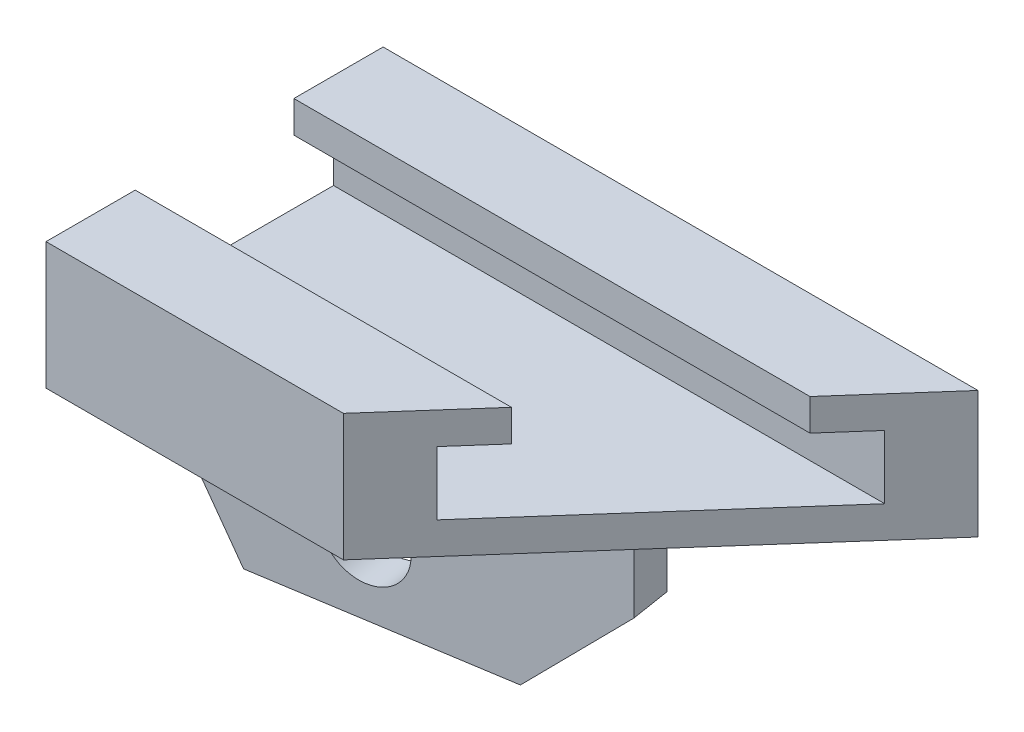
ISO-10303-21;
HEADER;
FILE_DESCRIPTION(('STEP AP214'),'2;1');
FILE_NAME('part.step','',(''),(''),'','','');
FILE_SCHEMA(('AUTOMOTIVE_DESIGN { 1 0 10303 214 1 1 1 1 }'));
ENDSEC;
DATA;
#1=APPLICATION_CONTEXT('core data for automotive mechanical design processes');
#2=APPLICATION_PROTOCOL_DEFINITION('international standard','automotive_design',2000,#1);
#3=PRODUCT_CONTEXT('',#1,'mechanical');
#4=PRODUCT('Part','Part','',(#3));
#5=PRODUCT_RELATED_PRODUCT_CATEGORY('part','',(#4));
#6=PRODUCT_DEFINITION_FORMATION('','',#4);
#7=PRODUCT_DEFINITION_CONTEXT('part definition',#1,'design');
#8=PRODUCT_DEFINITION('design','',#6,#7);
#9=PRODUCT_DEFINITION_SHAPE('','',#8);
#10=(LENGTH_UNIT() NAMED_UNIT(*) SI_UNIT(.MILLI.,.METRE.));
#11=(NAMED_UNIT(*) PLANE_ANGLE_UNIT() SI_UNIT($,.RADIAN.));
#12=(NAMED_UNIT(*) SI_UNIT($,.STERADIAN.) SOLID_ANGLE_UNIT());
#13=UNCERTAINTY_MEASURE_WITH_UNIT(LENGTH_MEASURE(1.E-05),#10,'distance_accuracy_value','');
#14=(GEOMETRIC_REPRESENTATION_CONTEXT(3) GLOBAL_UNCERTAINTY_ASSIGNED_CONTEXT((#13)) GLOBAL_UNIT_ASSIGNED_CONTEXT((#10,
#11,#12)) REPRESENTATION_CONTEXT('',''));
#15=CARTESIAN_POINT('',(0.,0.,0.));
#16=DIRECTION('',(0.,0.,1.));
#17=DIRECTION('',(1.,0.,0.));
#18=AXIS2_PLACEMENT_3D('',#15,#16,#17);
#19=CARTESIAN_POINT('',(32.7590302610631,-40.,-6.27670830561219));
#20=DIRECTION('',(-0.987688340595138,0.,0.156434465040231));
#21=DIRECTION('',(0.156434465040231,0.,0.987688340595138));
#22=AXIS2_PLACEMENT_3D('',#19,#20,#21);
#23=PLANE('',#22);
#24=DIRECTION('',(0.156434465040231,0.,0.987688340595138));
#25=VECTOR('',#24,1.);
#26=CARTESIAN_POINT('',(24.5251727273635,-15.,-58.2632387806263));
#27=LINE('',#26,#25);
#28=CARTESIAN_POINT('',(32.7590302610631,-15.,-6.27670830561219));
#29=VERTEX_POINT('',#28);
#30=CARTESIAN_POINT('',(34.3233749114654,-15.,3.60017510033917));
#31=VERTEX_POINT('',#30);
#32=EDGE_CURVE('E57',#29,#31,#27,.T.);
#33=ORIENTED_EDGE('',*,*,#32,.F.);
#34=DIRECTION('',(0.,1.,0.));
#35=VECTOR('',#34,1.);
#36=CARTESIAN_POINT('',(32.7590302610631,-40.,-6.27670830561219));
#37=LINE('',#36,#35);
#38=CARTESIAN_POINT('',(32.7590302610631,0.,-6.27670830561219));
#39=VERTEX_POINT('',#38);
#40=EDGE_CURVE('E275',#29,#39,#37,.T.);
#41=ORIENTED_EDGE('',*,*,#40,.T.);
#42=DIRECTION('',(0.156434465040231,0.,0.987688340595138));
#43=VECTOR('',#42,1.);
#44=CARTESIAN_POINT('',(32.7590302610631,0.,-6.27670830561219));
#45=LINE('',#44,#43);
#46=CARTESIAN_POINT('',(34.3233749114654,0.,3.60017510033917));
#47=VERTEX_POINT('',#46);
#48=EDGE_CURVE('E188',#39,#47,#45,.T.);
#49=ORIENTED_EDGE('',*,*,#48,.T.);
#50=DIRECTION('',(0.,1.,0.));
#51=VECTOR('',#50,1.);
#52=CARTESIAN_POINT('',(34.3233749114654,-40.,3.60017510033917));
#53=LINE('',#52,#51);
#54=EDGE_CURVE('E400',#31,#47,#53,.T.);
#55=ORIENTED_EDGE('',*,*,#54,.F.);
#56=EDGE_LOOP('',(#33,#41,#49,#55));
#57=FACE_BOUND('',#56,.T.);
#58=ADVANCED_FACE('F39',(#57),#23,.F.);
#59=CARTESIAN_POINT('',(-75.,-40.,10.7906453922011));
#60=DIRECTION('',(0.156434465040231,0.,0.987688340595138));
#61=DIRECTION('',(0.987688340595138,0.,-0.156434465040231));
#62=AXIS2_PLACEMENT_3D('',#59,#60,#61);
#63=PLANE('',#62);
#64=CARTESIAN_POINT('',(-25.6155829702431,-22.,2.96892214018953));
#65=DIRECTION('',(0.156434465040231,0.,0.987688340595138));
#66=DIRECTION('',(0.987688340595138,0.,-0.156434465040231));
#67=AXIS2_PLACEMENT_3D('',#64,#65,#66);
#68=CIRCLE('',#67,10.);
#69=CARTESIAN_POINT('',(-15.7386995642918,-22.,1.40457748978721));
#70=VERTEX_POINT('',#69);
#71=EDGE_CURVE('E190',#70,#70,#68,.T.);
#72=ORIENTED_EDGE('',*,*,#71,.T.);
#73=EDGE_LOOP('',(#72));
#74=FACE_BOUND('',#73,.T.);
#75=ORIENTED_EDGE('',*,*,#40,.F.);
#76=DIRECTION('',(-0.698401123333707,-0.707106781186551,0.110615871041237));
#77=VECTOR('',#76,1.);
#78=CARTESIAN_POINT('',(-33.4665891269071,-82.0511300640304,4.21239935629724));
#79=LINE('',#78,#77);
#80=CARTESIAN_POINT('',(8.06682174618494,-40.,-2.36584667960645));
#81=VERTEX_POINT('',#80);
#82=EDGE_CURVE('E403',#29,#81,#79,.T.);
#83=ORIENTED_EDGE('',*,*,#82,.T.);
#84=DIRECTION('',(0.987688340595138,0.,-0.156434465040231));
#85=VECTOR('',#84,1.);
#86=CARTESIAN_POINT('',(-75.,-40.,10.7906453922011));
#87=LINE('',#86,#85);
#88=CARTESIAN_POINT('',(-52.190314827278,-40.,7.17794617214064));
#89=VERTEX_POINT('',#88);
#90=EDGE_CURVE('E167',#89,#81,#87,.T.);
#91=ORIENTED_EDGE('',*,*,#90,.F.);
#92=DIRECTION('',(0.493844170297564,-0.866025403784441,-0.0782172325201147));
#93=VECTOR('',#92,1.);
#94=CARTESIAN_POINT('',(-57.8927361204584,-30.0000000000002,8.08112097715573));
#95=LINE('',#94,#93);
#96=CARTESIAN_POINT('',(-75.,0.,10.7906453922011));
#97=VERTEX_POINT('',#96);
#98=EDGE_CURVE('E159',#97,#89,#95,.T.);
#99=ORIENTED_EDGE('',*,*,#98,.F.);
#100=DIRECTION('',(0.987688340595138,0.,-0.156434465040231));
#101=VECTOR('',#100,1.);
#102=CARTESIAN_POINT('',(-75.,0.,10.7906453922011));
#103=LINE('',#102,#101);
#104=EDGE_CURVE('E175',#97,#39,#103,.T.);
#105=ORIENTED_EDGE('',*,*,#104,.T.);
#106=EDGE_LOOP('',(#75,#83,#91,#99,#105));
#107=FACE_BOUND('',#106,.T.);
#108=ADVANCED_FACE('F173',(#74,#107),#63,.F.);
#109=CARTESIAN_POINT('',(-73.4356553495977,-40.,20.6675287981525));
#110=DIRECTION('',(-0.156434465040231,0.,-0.987688340595138));
#111=DIRECTION('',(-0.987688340595138,0.,0.156434465040231));
#112=AXIS2_PLACEMENT_3D('',#109,#110,#111);
#113=PLANE('',#112);
#114=CARTESIAN_POINT('',(-24.0512383198408,-22.,12.8458055461409));
#115=DIRECTION('',(-0.156434465040231,0.,-0.987688340595138));
#116=DIRECTION('',(-0.987688340595138,0.,0.156434465040231));
#117=AXIS2_PLACEMENT_3D('',#114,#115,#116);
#118=CIRCLE('',#117,10.);
#119=CARTESIAN_POINT('',(-33.9281217257922,-22.,14.4101501965432));
#120=VERTEX_POINT('',#119);
#121=EDGE_CURVE('E43',#120,#120,#118,.T.);
#122=ORIENTED_EDGE('',*,*,#121,.T.);
#123=EDGE_LOOP('',(#122));
#124=FACE_BOUND('',#123,.T.);
#125=DIRECTION('',(-0.987688340595138,0.,0.156434465040231));
#126=VECTOR('',#125,1.);
#127=CARTESIAN_POINT('',(-73.4356553495977,-40.,20.6675287981525));
#128=LINE('',#127,#126);
#129=CARTESIAN_POINT('',(9.63116639658725,-40.,7.51103672634494));
#130=VERTEX_POINT('',#129);
#131=CARTESIAN_POINT('',(-50.6259701768757,-40.,17.054829578092));
#132=VERTEX_POINT('',#131);
#133=EDGE_CURVE('E395',#130,#132,#128,.T.);
#134=ORIENTED_EDGE('',*,*,#133,.F.);
#135=DIRECTION('',(0.698401123333707,0.707106781186551,-0.110615871041237));
#136=VECTOR('',#135,1.);
#137=CARTESIAN_POINT('',(-31.9022444765048,-82.0511300640304,14.0892827622486));
#138=LINE('',#137,#136);
#139=EDGE_CURVE('E177',#130,#31,#138,.T.);
#140=ORIENTED_EDGE('',*,*,#139,.T.);
#141=ORIENTED_EDGE('',*,*,#54,.T.);
#142=DIRECTION('',(-0.987688340595138,0.,0.156434465040231));
#143=VECTOR('',#142,1.);
#144=CARTESIAN_POINT('',(-73.4356553495977,0.,20.6675287981525));
#145=LINE('',#144,#143);
#146=CARTESIAN_POINT('',(-73.4356553495977,0.,20.6675287981525));
#147=VERTEX_POINT('',#146);
#148=EDGE_CURVE('E170',#47,#147,#145,.T.);
#149=ORIENTED_EDGE('',*,*,#148,.T.);
#150=DIRECTION('',(-0.493844170297564,0.866025403784442,0.0782172325201148));
#151=VECTOR('',#150,1.);
#152=CARTESIAN_POINT('',(-56.3283914700561,-30.0000000000002,17.9580043831071));
#153=LINE('',#152,#151);
#154=EDGE_CURVE('E161',#132,#147,#153,.T.);
#155=ORIENTED_EDGE('',*,*,#154,.F.);
#156=EDGE_LOOP('',(#134,#140,#141,#149,#155));
#157=FACE_BOUND('',#156,.T.);
#158=ADVANCED_FACE('F355',(#124,#157),#113,.F.);
#159=CARTESIAN_POINT('',(0.,-40.,0.));
#160=DIRECTION('',(0.,-1.,0.));
#161=DIRECTION('',(0.,0.,-1.));
#162=AXIS2_PLACEMENT_3D('',#159,#160,#161);
#163=PLANE('',#162);
#164=ORIENTED_EDGE('',*,*,#90,.T.);
#165=DIRECTION('',(0.156434465040231,0.,0.987688340595138));
#166=VECTOR('',#165,1.);
#167=CARTESIAN_POINT('',(-0.167035787514648,-40.,-54.3523771546206));
#168=LINE('',#167,#166);
#169=EDGE_CURVE('E11',#81,#130,#168,.T.);
#170=ORIENTED_EDGE('',*,*,#169,.T.);
#171=ORIENTED_EDGE('',*,*,#133,.T.);
#172=DIRECTION('',(0.156434465040231,0.,0.987688340595138));
#173=VECTOR('',#172,1.);
#174=CARTESIAN_POINT('',(-60.4241723609776,-40.,-44.8085843028735));
#175=LINE('',#174,#173);
#176=EDGE_CURVE('E48',#89,#132,#175,.T.);
#177=ORIENTED_EDGE('',*,*,#176,.F.);
#178=EDGE_LOOP('',(#164,#170,#171,#177));
#179=FACE_BOUND('',#178,.T.);
#180=ADVANCED_FACE('F383',(#179),#163,.T.);
#181=CARTESIAN_POINT('',(0.,0.,0.));
#182=DIRECTION('',(0.,1.,0.));
#183=DIRECTION('',(0.,0.,1.));
#184=AXIS2_PLACEMENT_3D('',#181,#182,#183);
#185=PLANE('',#184);
#186=ORIENTED_EDGE('',*,*,#104,.F.);
#187=DIRECTION('',(0.,0.,1.));
#188=VECTOR('',#187,1.);
#189=CARTESIAN_POINT('',(-75.,0.,-42.5));
#190=LINE('',#189,#188);
#191=CARTESIAN_POINT('',(-75.,0.,-42.5));
#192=VERTEX_POINT('',#191);
#193=EDGE_CURVE('E186',#192,#97,#190,.T.);
#194=ORIENTED_EDGE('',*,*,#193,.F.);
#195=DIRECTION('',(-1.,0.,0.));
#196=VECTOR('',#195,1.);
#197=CARTESIAN_POINT('',(-75.,0.,-42.5));
#198=LINE('',#197,#196);
#199=CARTESIAN_POINT('',(75.,0.,-42.5));
#200=VERTEX_POINT('',#199);
#201=EDGE_CURVE('E216',#200,#192,#198,.T.);
#202=ORIENTED_EDGE('',*,*,#201,.F.);
#203=DIRECTION('',(0.661621637086846,0.,-0.749837855365093));
#204=VECTOR('',#203,1.);
#205=CARTESIAN_POINT('',(0.,0.,42.5));
#206=LINE('',#205,#204);
#207=EDGE_CURVE('E210',#47,#200,#206,.T.);
#208=ORIENTED_EDGE('',*,*,#207,.F.);
#209=ORIENTED_EDGE('',*,*,#48,.F.);
#210=EDGE_LOOP('',(#186,#194,#202,#208,#209));
#211=FACE_BOUND('',#210,.T.);
#212=ADVANCED_FACE('F181',(#211),#185,.F.);
#213=DIRECTION('',(-0.156434465040231,0.,-0.987688340595138));
#214=VECTOR('',#213,1.);
#215=CARTESIAN_POINT('',(-75.,0.,10.7906453922011));
#216=LINE('',#215,#214);
#217=EDGE_CURVE('E160',#147,#97,#216,.T.);
#218=ORIENTED_EDGE('',*,*,#217,.F.);
#219=ORIENTED_EDGE('',*,*,#148,.F.);
#220=CARTESIAN_POINT('',(0.,0.,42.5));
#221=VERTEX_POINT('',#220);
#222=EDGE_CURVE('E213',#221,#47,#206,.T.);
#223=ORIENTED_EDGE('',*,*,#222,.F.);
#224=DIRECTION('',(1.,0.,0.));
#225=VECTOR('',#224,1.);
#226=CARTESIAN_POINT('',(-75.,0.,42.5));
#227=LINE('',#226,#225);
#228=CARTESIAN_POINT('',(-75.,0.,42.5));
#229=VERTEX_POINT('',#228);
#230=EDGE_CURVE('E198',#229,#221,#227,.T.);
#231=ORIENTED_EDGE('',*,*,#230,.F.);
#232=EDGE_CURVE('E192',#97,#229,#190,.T.);
#233=ORIENTED_EDGE('',*,*,#232,.F.);
#234=EDGE_LOOP('',(#218,#219,#223,#231,#233));
#235=FACE_BOUND('',#234,.T.);
#236=ADVANCED_FACE('F193',(#235),#185,.F.);
#237=CARTESIAN_POINT('',(-75.,32.,-42.5));
#238=DIRECTION('',(1.,0.,0.));
#239=DIRECTION('',(0.,0.,-1.));
#240=AXIS2_PLACEMENT_3D('',#237,#238,#239);
#241=PLANE('',#240);
#242=DIRECTION('',(0.,1.,0.));
#243=VECTOR('',#242,1.);
#244=CARTESIAN_POINT('',(-75.,32.,20.));
#245=LINE('',#244,#243);
#246=CARTESIAN_POINT('',(-75.,24.,20.));
#247=VERTEX_POINT('',#246);
#248=CARTESIAN_POINT('',(-75.,32.,20.));
#249=VERTEX_POINT('',#248);
#250=EDGE_CURVE('E270',#247,#249,#245,.T.);
#251=ORIENTED_EDGE('',*,*,#250,.F.);
#252=DIRECTION('',(0.,0.,-1.));
#253=VECTOR('',#252,1.);
#254=CARTESIAN_POINT('',(-75.,24.,20.));
#255=LINE('',#254,#253);
#256=CARTESIAN_POINT('',(-75.,24.,30.));
#257=VERTEX_POINT('',#256);
#258=EDGE_CURVE('E267',#257,#247,#255,.T.);
#259=ORIENTED_EDGE('',*,*,#258,.F.);
#260=DIRECTION('',(0.,1.,0.));
#261=VECTOR('',#260,1.);
#262=CARTESIAN_POINT('',(-75.,8.,30.));
#263=LINE('',#262,#261);
#264=CARTESIAN_POINT('',(-75.,8.,30.));
#265=VERTEX_POINT('',#264);
#266=EDGE_CURVE('E253',#265,#257,#263,.T.);
#267=ORIENTED_EDGE('',*,*,#266,.F.);
#268=DIRECTION('',(0.,0.,1.));
#269=VECTOR('',#268,1.);
#270=CARTESIAN_POINT('',(-75.,8.,-30.));
#271=LINE('',#270,#269);
#272=CARTESIAN_POINT('',(-75.,8.,-30.));
#273=VERTEX_POINT('',#272);
#274=EDGE_CURVE('E254',#273,#265,#271,.T.);
#275=ORIENTED_EDGE('',*,*,#274,.F.);
#276=DIRECTION('',(0.,-1.,0.));
#277=VECTOR('',#276,1.);
#278=CARTESIAN_POINT('',(-75.,8.,-30.));
#279=LINE('',#278,#277);
#280=CARTESIAN_POINT('',(-75.,24.,-30.));
#281=VERTEX_POINT('',#280);
#282=EDGE_CURVE('E256',#281,#273,#279,.T.);
#283=ORIENTED_EDGE('',*,*,#282,.F.);
#284=DIRECTION('',(0.,0.,-1.));
#285=VECTOR('',#284,1.);
#286=CARTESIAN_POINT('',(-75.,24.,-30.));
#287=LINE('',#286,#285);
#288=CARTESIAN_POINT('',(-75.,24.,-20.));
#289=VERTEX_POINT('',#288);
#290=EDGE_CURVE('E261',#289,#281,#287,.T.);
#291=ORIENTED_EDGE('',*,*,#290,.F.);
#292=DIRECTION('',(0.,-1.,0.));
#293=VECTOR('',#292,1.);
#294=CARTESIAN_POINT('',(-75.,32.,-20.));
#295=LINE('',#294,#293);
#296=CARTESIAN_POINT('',(-75.,32.,-20.));
#297=VERTEX_POINT('',#296);
#298=EDGE_CURVE('E262',#297,#289,#295,.T.);
#299=ORIENTED_EDGE('',*,*,#298,.F.);
#300=DIRECTION('',(0.,0.,1.));
#301=VECTOR('',#300,1.);
#302=CARTESIAN_POINT('',(-75.,32.,0.));
#303=LINE('',#302,#301);
#304=CARTESIAN_POINT('',(-75.,32.,-42.5));
#305=VERTEX_POINT('',#304);
#306=EDGE_CURVE('E235',#305,#297,#303,.T.);
#307=ORIENTED_EDGE('',*,*,#306,.F.);
#308=DIRECTION('',(0.,-1.,0.));
#309=VECTOR('',#308,1.);
#310=CARTESIAN_POINT('',(-75.,32.,-42.5));
#311=LINE('',#310,#309);
#312=EDGE_CURVE('E206',#305,#192,#311,.T.);
#313=ORIENTED_EDGE('',*,*,#312,.T.);
#314=ORIENTED_EDGE('',*,*,#193,.T.);
#315=ORIENTED_EDGE('',*,*,#232,.T.);
#316=DIRECTION('',(0.,-1.,0.));
#317=VECTOR('',#316,1.);
#318=CARTESIAN_POINT('',(-75.,32.,42.5));
#319=LINE('',#318,#317);
#320=CARTESIAN_POINT('',(-75.,32.,42.5));
#321=VERTEX_POINT('',#320);
#322=EDGE_CURVE('E223',#321,#229,#319,.T.);
#323=ORIENTED_EDGE('',*,*,#322,.F.);
#324=DIRECTION('',(0.,0.,1.));
#325=VECTOR('',#324,1.);
#326=CARTESIAN_POINT('',(-75.,32.,0.));
#327=LINE('',#326,#325);
#328=EDGE_CURVE('E217',#249,#321,#327,.T.);
#329=ORIENTED_EDGE('',*,*,#328,.F.);
#330=EDGE_LOOP('',(#251,#259,#267,#275,#283,#291,#299,#307,#313,#314,#315,#323,#329));
#331=FACE_BOUND('',#330,.T.);
#332=ADVANCED_FACE('F41',(#331),#241,.F.);
#333=CARTESIAN_POINT('',(0.,32.,0.));
#334=DIRECTION('',(0.,1.,0.));
#335=DIRECTION('',(0.,0.,1.));
#336=AXIS2_PLACEMENT_3D('',#333,#334,#335);
#337=PLANE('',#336);
#338=DIRECTION('',(0.661621637086846,0.,-0.749837855365093));
#339=VECTOR('',#338,1.);
#340=CARTESIAN_POINT('',(0.,32.,42.5));
#341=LINE('',#340,#339);
#342=CARTESIAN_POINT('',(0.,32.,42.5));
#343=VERTEX_POINT('',#342);
#344=CARTESIAN_POINT('',(19.8529411764706,32.,20.));
#345=VERTEX_POINT('',#344);
#346=EDGE_CURVE('E209',#343,#345,#341,.T.);
#347=ORIENTED_EDGE('',*,*,#346,.T.);
#348=DIRECTION('',(-1.,0.,0.));
#349=VECTOR('',#348,1.);
#350=CARTESIAN_POINT('',(75.,32.,20.));
#351=LINE('',#350,#349);
#352=EDGE_CURVE('E233',#345,#249,#351,.T.);
#353=ORIENTED_EDGE('',*,*,#352,.T.);
#354=ORIENTED_EDGE('',*,*,#328,.T.);
#355=DIRECTION('',(1.,0.,0.));
#356=VECTOR('',#355,1.);
#357=CARTESIAN_POINT('',(-75.,32.,42.5));
#358=LINE('',#357,#356);
#359=EDGE_CURVE('E228',#321,#343,#358,.T.);
#360=ORIENTED_EDGE('',*,*,#359,.T.);
#361=EDGE_LOOP('',(#347,#353,#354,#360));
#362=FACE_BOUND('',#361,.T.);
#363=ADVANCED_FACE('F276',(#362),#337,.T.);
#364=CARTESIAN_POINT('',(-75.,32.,42.5));
#365=DIRECTION('',(0.,0.,-1.));
#366=DIRECTION('',(-1.,0.,0.));
#367=AXIS2_PLACEMENT_3D('',#364,#365,#366);
#368=PLANE('',#367);
#369=ORIENTED_EDGE('',*,*,#230,.T.);
#370=DIRECTION('',(0.,-1.,0.));
#371=VECTOR('',#370,1.);
#372=CARTESIAN_POINT('',(0.,32.,42.5));
#373=LINE('',#372,#371);
#374=EDGE_CURVE('E225',#343,#221,#373,.T.);
#375=ORIENTED_EDGE('',*,*,#374,.F.);
#376=ORIENTED_EDGE('',*,*,#359,.F.);
#377=ORIENTED_EDGE('',*,*,#322,.T.);
#378=EDGE_LOOP('',(#369,#375,#376,#377));
#379=FACE_BOUND('',#378,.T.);
#380=ADVANCED_FACE('F282',(#379),#368,.F.);
#381=CARTESIAN_POINT('',(0.,32.,42.5));
#382=DIRECTION('',(-0.749837855365093,0.,-0.661621637086846));
#383=DIRECTION('',(-0.661621637086846,0.,0.749837855365093));
#384=AXIS2_PLACEMENT_3D('',#381,#382,#383);
#385=PLANE('',#384);
#386=CARTESIAN_POINT('',(55.1470588235294,32.,-20.));
#387=VERTEX_POINT('',#386);
#388=CARTESIAN_POINT('',(75.,32.,-42.5));
#389=VERTEX_POINT('',#388);
#390=EDGE_CURVE('E231',#387,#389,#341,.T.);
#391=ORIENTED_EDGE('',*,*,#390,.F.);
#392=DIRECTION('',(0.,-1.,0.));
#393=VECTOR('',#392,1.);
#394=CARTESIAN_POINT('',(55.1470588235294,32.,-20.));
#395=LINE('',#394,#393);
#396=CARTESIAN_POINT('',(55.1470588235294,24.,-20.));
#397=VERTEX_POINT('',#396);
#398=EDGE_CURVE('E199',#387,#397,#395,.T.);
#399=ORIENTED_EDGE('',*,*,#398,.T.);
#400=DIRECTION('',(0.661621637086846,0.,-0.749837855365093));
#401=VECTOR('',#400,1.);
#402=CARTESIAN_POINT('',(0.,24.,42.5));
#403=LINE('',#402,#401);
#404=CARTESIAN_POINT('',(63.9705882352941,24.,-30.));
#405=VERTEX_POINT('',#404);
#406=EDGE_CURVE('E247',#397,#405,#403,.T.);
#407=ORIENTED_EDGE('',*,*,#406,.T.);
#408=DIRECTION('',(0.,-1.,0.));
#409=VECTOR('',#408,1.);
#410=CARTESIAN_POINT('',(63.9705882352941,32.,-30.));
#411=LINE('',#410,#409);
#412=CARTESIAN_POINT('',(63.9705882352941,8.,-30.));
#413=VERTEX_POINT('',#412);
#414=EDGE_CURVE('E245',#405,#413,#411,.T.);
#415=ORIENTED_EDGE('',*,*,#414,.T.);
#416=DIRECTION('',(-0.661621637086846,0.,0.749837855365093));
#417=VECTOR('',#416,1.);
#418=CARTESIAN_POINT('',(0.,8.,42.5));
#419=LINE('',#418,#417);
#420=CARTESIAN_POINT('',(11.0294117647059,8.,30.));
#421=VERTEX_POINT('',#420);
#422=EDGE_CURVE('E242',#413,#421,#419,.T.);
#423=ORIENTED_EDGE('',*,*,#422,.T.);
#424=DIRECTION('',(0.,1.,0.));
#425=VECTOR('',#424,1.);
#426=CARTESIAN_POINT('',(11.0294117647059,32.,30.));
#427=LINE('',#426,#425);
#428=CARTESIAN_POINT('',(11.0294117647059,24.,30.));
#429=VERTEX_POINT('',#428);
#430=EDGE_CURVE('E236',#421,#429,#427,.T.);
#431=ORIENTED_EDGE('',*,*,#430,.T.);
#432=DIRECTION('',(0.661621637086846,0.,-0.749837855365093));
#433=VECTOR('',#432,1.);
#434=CARTESIAN_POINT('',(0.,24.,42.5));
#435=LINE('',#434,#433);
#436=CARTESIAN_POINT('',(19.8529411764706,24.,20.));
#437=VERTEX_POINT('',#436);
#438=EDGE_CURVE('E234',#429,#437,#435,.T.);
#439=ORIENTED_EDGE('',*,*,#438,.T.);
#440=DIRECTION('',(0.,1.,0.));
#441=VECTOR('',#440,1.);
#442=CARTESIAN_POINT('',(19.8529411764706,32.,20.));
#443=LINE('',#442,#441);
#444=EDGE_CURVE('E287',#437,#345,#443,.T.);
#445=ORIENTED_EDGE('',*,*,#444,.T.);
#446=ORIENTED_EDGE('',*,*,#346,.F.);
#447=ORIENTED_EDGE('',*,*,#374,.T.);
#448=ORIENTED_EDGE('',*,*,#222,.T.);
#449=ORIENTED_EDGE('',*,*,#207,.T.);
#450=DIRECTION('',(0.,-1.,0.));
#451=VECTOR('',#450,1.);
#452=CARTESIAN_POINT('',(75.,32.,-42.5));
#453=LINE('',#452,#451);
#454=EDGE_CURVE('E218',#389,#200,#453,.T.);
#455=ORIENTED_EDGE('',*,*,#454,.F.);
#456=EDGE_LOOP('',(#391,#399,#407,#415,#423,#431,#439,#445,#446,#447,#448,#449,#455));
#457=FACE_BOUND('',#456,.T.);
#458=ADVANCED_FACE('F290',(#457),#385,.F.);
#459=CARTESIAN_POINT('',(-75.,32.,-42.5));
#460=DIRECTION('',(0.,0.,1.));
#461=DIRECTION('',(1.,0.,0.));
#462=AXIS2_PLACEMENT_3D('',#459,#460,#461);
#463=PLANE('',#462);
#464=ORIENTED_EDGE('',*,*,#201,.T.);
#465=ORIENTED_EDGE('',*,*,#312,.F.);
#466=DIRECTION('',(-1.,0.,0.));
#467=VECTOR('',#466,1.);
#468=CARTESIAN_POINT('',(-75.,32.,-42.5));
#469=LINE('',#468,#467);
#470=EDGE_CURVE('E226',#389,#305,#469,.T.);
#471=ORIENTED_EDGE('',*,*,#470,.F.);
#472=ORIENTED_EDGE('',*,*,#454,.T.);
#473=EDGE_LOOP('',(#464,#465,#471,#472));
#474=FACE_BOUND('',#473,.T.);
#475=ADVANCED_FACE('F296',(#474),#463,.F.);
#476=DIRECTION('',(-1.,0.,0.));
#477=VECTOR('',#476,1.);
#478=CARTESIAN_POINT('',(75.,32.,-20.));
#479=LINE('',#478,#477);
#480=EDGE_CURVE('E239',#387,#297,#479,.T.);
#481=ORIENTED_EDGE('',*,*,#480,.F.);
#482=ORIENTED_EDGE('',*,*,#390,.T.);
#483=ORIENTED_EDGE('',*,*,#470,.T.);
#484=ORIENTED_EDGE('',*,*,#306,.T.);
#485=EDGE_LOOP('',(#481,#482,#483,#484));
#486=FACE_BOUND('',#485,.T.);
#487=ADVANCED_FACE('F295',(#486),#337,.T.);
#488=CARTESIAN_POINT('',(75.,24.,20.));
#489=DIRECTION('',(0.,1.,0.));
#490=DIRECTION('',(0.,0.,1.));
#491=AXIS2_PLACEMENT_3D('',#488,#489,#490);
#492=PLANE('',#491);
#493=DIRECTION('',(-1.,0.,0.));
#494=VECTOR('',#493,1.);
#495=CARTESIAN_POINT('',(75.,24.,30.));
#496=LINE('',#495,#494);
#497=EDGE_CURVE('E312',#429,#257,#496,.T.);
#498=ORIENTED_EDGE('',*,*,#497,.T.);
#499=ORIENTED_EDGE('',*,*,#258,.T.);
#500=DIRECTION('',(-1.,0.,0.));
#501=VECTOR('',#500,1.);
#502=CARTESIAN_POINT('',(75.,24.,20.));
#503=LINE('',#502,#501);
#504=EDGE_CURVE('E255',#437,#247,#503,.T.);
#505=ORIENTED_EDGE('',*,*,#504,.F.);
#506=ORIENTED_EDGE('',*,*,#438,.F.);
#507=EDGE_LOOP('',(#498,#499,#505,#506));
#508=FACE_BOUND('',#507,.T.);
#509=ADVANCED_FACE('F339',(#508),#492,.F.);
#510=CARTESIAN_POINT('',(75.,8.,30.));
#511=DIRECTION('',(0.,0.,1.));
#512=DIRECTION('',(1.,0.,0.));
#513=AXIS2_PLACEMENT_3D('',#510,#511,#512);
#514=PLANE('',#513);
#515=DIRECTION('',(-1.,0.,0.));
#516=VECTOR('',#515,1.);
#517=CARTESIAN_POINT('',(75.,8.,30.));
#518=LINE('',#517,#516);
#519=EDGE_CURVE('E311',#421,#265,#518,.T.);
#520=ORIENTED_EDGE('',*,*,#519,.T.);
#521=ORIENTED_EDGE('',*,*,#266,.T.);
#522=ORIENTED_EDGE('',*,*,#497,.F.);
#523=ORIENTED_EDGE('',*,*,#430,.F.);
#524=EDGE_LOOP('',(#520,#521,#522,#523));
#525=FACE_BOUND('',#524,.T.);
#526=ADVANCED_FACE('F328',(#525),#514,.F.);
#527=CARTESIAN_POINT('',(75.,8.,-30.));
#528=DIRECTION('',(0.,-1.,0.));
#529=DIRECTION('',(0.,0.,-1.));
#530=AXIS2_PLACEMENT_3D('',#527,#528,#529);
#531=PLANE('',#530);
#532=DIRECTION('',(-1.,0.,0.));
#533=VECTOR('',#532,1.);
#534=CARTESIAN_POINT('',(75.,8.,-30.));
#535=LINE('',#534,#533);
#536=EDGE_CURVE('E313',#413,#273,#535,.T.);
#537=ORIENTED_EDGE('',*,*,#536,.T.);
#538=ORIENTED_EDGE('',*,*,#274,.T.);
#539=ORIENTED_EDGE('',*,*,#519,.F.);
#540=ORIENTED_EDGE('',*,*,#422,.F.);
#541=EDGE_LOOP('',(#537,#538,#539,#540));
#542=FACE_BOUND('',#541,.T.);
#543=ADVANCED_FACE('F322',(#542),#531,.F.);
#544=CARTESIAN_POINT('',(75.,8.,-30.));
#545=DIRECTION('',(0.,0.,-1.));
#546=DIRECTION('',(-1.,0.,0.));
#547=AXIS2_PLACEMENT_3D('',#544,#545,#546);
#548=PLANE('',#547);
#549=DIRECTION('',(-1.,0.,0.));
#550=VECTOR('',#549,1.);
#551=CARTESIAN_POINT('',(75.,24.,-30.));
#552=LINE('',#551,#550);
#553=EDGE_CURVE('E310',#405,#281,#552,.T.);
#554=ORIENTED_EDGE('',*,*,#553,.T.);
#555=ORIENTED_EDGE('',*,*,#282,.T.);
#556=ORIENTED_EDGE('',*,*,#536,.F.);
#557=ORIENTED_EDGE('',*,*,#414,.F.);
#558=EDGE_LOOP('',(#554,#555,#556,#557));
#559=FACE_BOUND('',#558,.T.);
#560=ADVANCED_FACE('F319',(#559),#548,.F.);
#561=CARTESIAN_POINT('',(75.,24.,-30.));
#562=DIRECTION('',(0.,1.,0.));
#563=DIRECTION('',(0.,0.,1.));
#564=AXIS2_PLACEMENT_3D('',#561,#562,#563);
#565=PLANE('',#564);
#566=DIRECTION('',(-1.,0.,0.));
#567=VECTOR('',#566,1.);
#568=CARTESIAN_POINT('',(75.,24.,-20.));
#569=LINE('',#568,#567);
#570=EDGE_CURVE('E302',#397,#289,#569,.T.);
#571=ORIENTED_EDGE('',*,*,#570,.T.);
#572=ORIENTED_EDGE('',*,*,#290,.T.);
#573=ORIENTED_EDGE('',*,*,#553,.F.);
#574=ORIENTED_EDGE('',*,*,#406,.F.);
#575=EDGE_LOOP('',(#571,#572,#573,#574));
#576=FACE_BOUND('',#575,.T.);
#577=ADVANCED_FACE('F318',(#576),#565,.F.);
#578=CARTESIAN_POINT('',(75.,32.,-20.));
#579=DIRECTION('',(0.,0.,-1.));
#580=DIRECTION('',(-1.,0.,0.));
#581=AXIS2_PLACEMENT_3D('',#578,#579,#580);
#582=PLANE('',#581);
#583=ORIENTED_EDGE('',*,*,#480,.T.);
#584=ORIENTED_EDGE('',*,*,#298,.T.);
#585=ORIENTED_EDGE('',*,*,#570,.F.);
#586=ORIENTED_EDGE('',*,*,#398,.F.);
#587=EDGE_LOOP('',(#583,#584,#585,#586));
#588=FACE_BOUND('',#587,.T.);
#589=ADVANCED_FACE('F305',(#588),#582,.F.);
#590=CARTESIAN_POINT('',(75.,32.,20.));
#591=DIRECTION('',(0.,0.,1.));
#592=DIRECTION('',(0.,-1.,0.));
#593=AXIS2_PLACEMENT_3D('',#590,#591,#592);
#594=PLANE('',#593);
#595=ORIENTED_EDGE('',*,*,#504,.T.);
#596=ORIENTED_EDGE('',*,*,#250,.T.);
#597=ORIENTED_EDGE('',*,*,#352,.F.);
#598=ORIENTED_EDGE('',*,*,#444,.F.);
#599=EDGE_LOOP('',(#595,#596,#597,#598));
#600=FACE_BOUND('',#599,.T.);
#601=ADVANCED_FACE('F337',(#600),#594,.F.);
#602=CARTESIAN_POINT('',(-33.8494405039427,-22.,-49.0176083348246));
#603=DIRECTION('',(0.156434465040231,0.,0.987688340595138));
#604=DIRECTION('',(0.987688340595138,0.,-0.156434465040231));
#605=AXIS2_PLACEMENT_3D('',#602,#603,#604);
#606=CYLINDRICAL_SURFACE('',#605,10.);
#607=ORIENTED_EDGE('',*,*,#121,.F.);
#608=EDGE_LOOP('',(#607));
#609=FACE_BOUND('',#608,.T.);
#610=ORIENTED_EDGE('',*,*,#71,.F.);
#611=EDGE_LOOP('',(#610));
#612=FACE_BOUND('',#611,.T.);
#613=ADVANCED_FACE('F369',(#609,#612),#606,.F.);
#614=CARTESIAN_POINT('',(-64.5258910926249,-32.8070577027472,-44.1589358771929));
#615=DIRECTION('',(-0.855363193977089,-0.499999999999995,0.135476220752269));
#616=DIRECTION('',(0.504652595083946,-0.86332251115967,0.));
#617=AXIS2_PLACEMENT_3D('',#614,#615,#616);
#618=PLANE('',#617);
#619=ORIENTED_EDGE('',*,*,#98,.T.);
#620=ORIENTED_EDGE('',*,*,#176,.T.);
#621=ORIENTED_EDGE('',*,*,#154,.T.);
#622=ORIENTED_EDGE('',*,*,#217,.T.);
#623=EDGE_LOOP('',(#619,#620,#621,#622));
#624=FACE_BOUND('',#623,.T.);
#625=ADVANCED_FACE('F157',(#624),#618,.T.);
#626=CARTESIAN_POINT('',(15.4692530334458,-24.1688028720286,-56.8289220082812));
#627=DIRECTION('',(-0.698401123333714,0.707106781186544,0.110615871041238));
#628=DIRECTION('',(-0.711472923612858,-0.702713511301563,0.));
#629=AXIS2_PLACEMENT_3D('',#626,#627,#628);
#630=PLANE('',#629);
#631=ORIENTED_EDGE('',*,*,#32,.T.);
#632=ORIENTED_EDGE('',*,*,#139,.F.);
#633=ORIENTED_EDGE('',*,*,#169,.F.);
#634=ORIENTED_EDGE('',*,*,#82,.F.);
#635=EDGE_LOOP('',(#631,#632,#633,#634));
#636=FACE_BOUND('',#635,.T.);
#637=ADVANCED_FACE('F377',(#636),#630,.F.);
#638=CLOSED_SHELL('',(#58,#108,#158,#180,#212,#236,#332,#363,#380,#458,#475,#487,#509,#526,#543,
#560,#577,#589,#601,#613,#625,#637));
#639=MANIFOLD_SOLID_BREP('B2',#638);
#640=ADVANCED_BREP_SHAPE_REPRESENTATION('',(#18,#639),#14);
#641=SHAPE_DEFINITION_REPRESENTATION(#9,#640);
ENDSEC;
END-ISO-10303-21;
